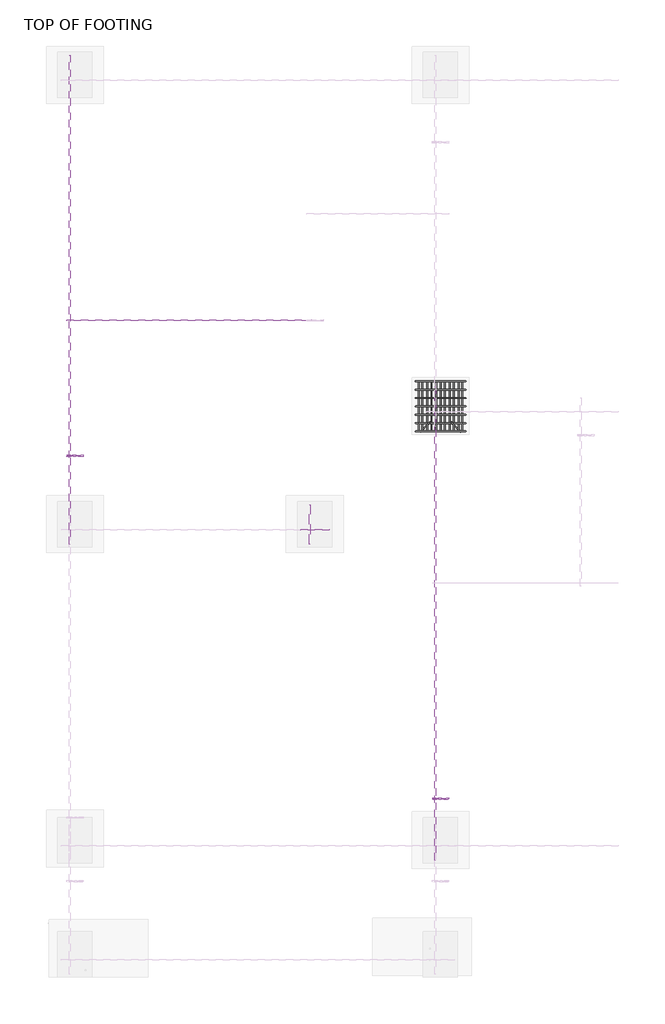
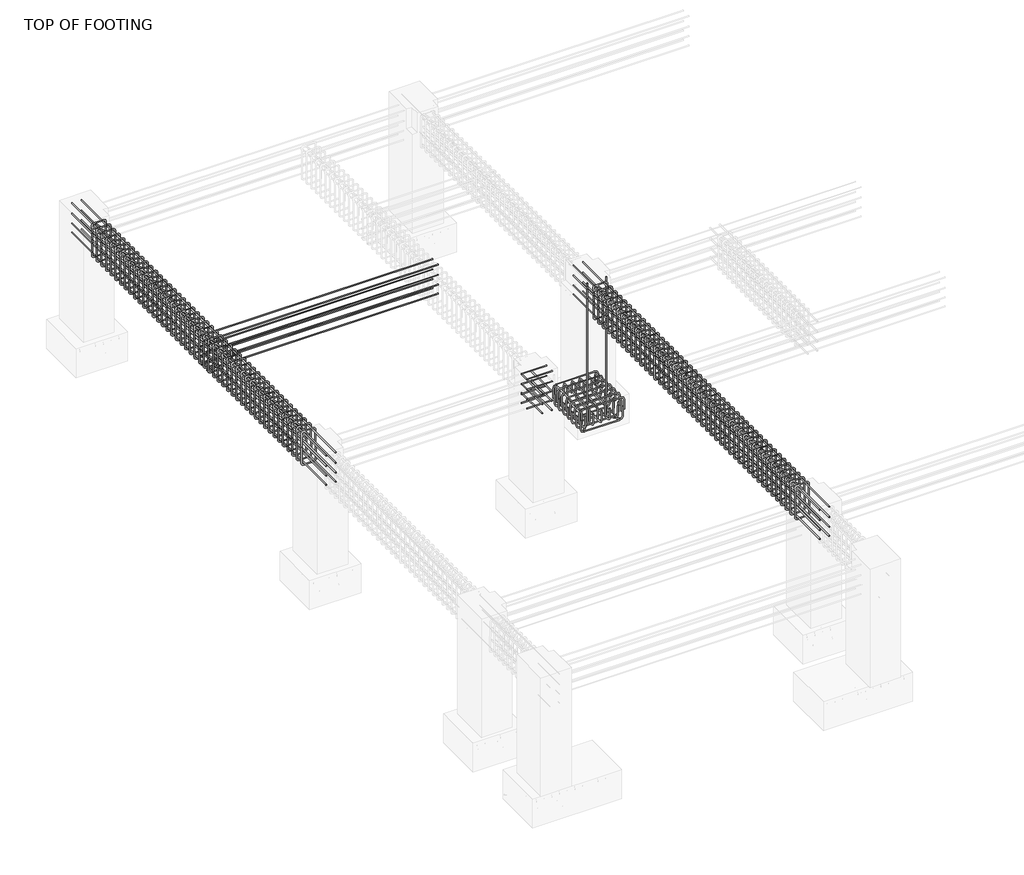
# One storey, part 5 of 8: 27 reinforcing bars.
"""IFC4 building model written with IfcOpenShell, lengths in millimetres."""

from ifc_helpers import new_model, si_unit, point, frame, origin, place, context, project, spatial, polyline, circle_curve, trimmed, segment, composite_curve, source, transform, mapped, element, save
from ifc_brep_helpers import swept_disk

model = new_model("IFC4")

# Units and contexts
model_context = context("Model", 3, world=origin())
ifc_project = project(units=[si_unit("LENGTHUNIT", "METRE", prefix="MILLI")], contexts=[model_context])

# Site, building, storey
site = spatial("IfcSite", under=ifc_project)
building = spatial("IfcBuilding", under=site)
storey = spatial("IfcBuildingStorey", under=building, Name="TOP OF FOOTING", Elevation=-1828.8)

# Reinforcing bars
placement = place(None, origin())
reinforcing_bar_shape = source(origin(), model_context, "Body", "SolidModel", [
    swept_disk(composite_curve([segment(polyline([(-1395.5877818, 5545.6420243, -2021.245224), (-1395.5877818, 5545.6420243, -2168.545224)]), True, "CONTINUOUS"), segment(trimmed(circle_curve(frame((-1441.9377818, 5545.6420243, -2168.545224), z_axis=(0.0, 1.0, 0.0), x_axis=(46.350000000000136, 0.0, 0.0)), 46.35), [point((-1395.5877818, 5545.6420243, -2168.545224))], [point((-1441.9377818, 5545.6420243, -2214.895224))], True, "CARTESIAN"), True, "CONTINUOUS"), segment(polyline([(-1441.9377818, 5545.6420243, -2214.895224), (-1962.8758647, 5545.6420243, -2214.895224)]), True, "CONTINUOUS"), segment(trimmed(circle_curve(frame((-1962.8758647, 5545.6420243, -2168.545224), z_axis=(0.0, 1.0, 0.0), x_axis=(0.0, 0.0, -46.34999999999991)), 46.35), [point((-1962.8758647, 5545.6420243, -2214.895224))], [point((-2009.2258647, 5545.6420243, -2168.545224))], True, "CARTESIAN"), True, "CONTINUOUS"), segment(polyline([(-2009.2258647, 5545.6420243, -2168.545224), (-2009.2258647, 5545.6420243, -2021.245224)]), True, "CONTINUOUS")], self_intersect=False), 6.35),
])
element("IfcReinforcingBar", 1, at=placement, inside=storey, context=model_context, shape_type="MappedRepresentation", body=[
    mapped(reinforcing_bar_shape, transform((0.0, 0.0, 0.0), x_axis=(1.0, 0.0, 0.0), y_axis=(0.0, 1.0, 0.0), z_axis=(0.0, 0.0, 1.0))),
    mapped(reinforcing_bar_shape, transform((0.0, -109.55, 0.0), x_axis=(1.0, 0.0, 0.0), y_axis=(0.0, 1.0, 0.0), z_axis=(0.0, 0.0, 1.0))),
    mapped(reinforcing_bar_shape, transform((0.0, -219.1, 0.0), x_axis=(1.0, 0.0, 0.0), y_axis=(0.0, 1.0, 0.0), z_axis=(0.0, 0.0, 1.0))),
    mapped(reinforcing_bar_shape, transform((0.0, -328.65, 0.0), x_axis=(1.0, 0.0, 0.0), y_axis=(0.0, 1.0, 0.0), z_axis=(0.0, 0.0, 1.0))),
    mapped(reinforcing_bar_shape, transform((0.0, -438.2, 0.0), x_axis=(1.0, 0.0, 0.0), y_axis=(0.0, 1.0, 0.0), z_axis=(0.0, 0.0, 1.0))),
    mapped(reinforcing_bar_shape, transform((0.0, -547.75, 0.0), x_axis=(1.0, 0.0, 0.0), y_axis=(0.0, 1.0, 0.0), z_axis=(0.0, 0.0, 1.0))),
    mapped(reinforcing_bar_shape, transform((0.0, -657.3, 0.0), x_axis=(1.0, 0.0, 0.0), y_axis=(0.0, 1.0, 0.0), z_axis=(0.0, 0.0, 1.0))),
])
reinforcing_bar_2_shape = source(origin(), model_context, "Body", "SolidModel", [
    swept_disk(composite_curve([segment(polyline([(-2031.1461367, 5545.6420243, -2068.8), (-2031.1461367, 5545.6420243, -1921.5)]), True, "CONTINUOUS"), segment(trimmed(circle_curve(frame((-1984.7961367, 5545.6420243, -1921.5), z_axis=(0.0, 1.0, 0.0), x_axis=(-46.34999999999991, 0.0, 0.0)), 46.35), [point((-2031.1461367, 5545.6420243, -1921.5))], [point((-1984.7961367, 5545.6420243, -1875.15))], True, "CARTESIAN"), True, "CONTINUOUS"), segment(polyline([(-1984.7961367, 5545.6420243, -1875.15), (-1420.1961367, 5545.6420243, -1875.15)]), True, "CONTINUOUS"), segment(trimmed(circle_curve(frame((-1420.1961367, 5545.6420243, -1921.5), z_axis=(0.0, 1.0, 0.0), x_axis=(0.0, 0.0, 46.34999999999991)), 46.35), [point((-1420.1961367, 5545.6420243, -1875.15))], [point((-1373.8461367, 5545.6420243, -1921.5))], True, "CARTESIAN"), True, "CONTINUOUS"), segment(polyline([(-1373.8461367, 5545.6420243, -1921.5), (-1373.8461367, 5545.6420243, -2068.8)]), True, "CONTINUOUS")], self_intersect=False), 6.35),
])
element("IfcReinforcingBar", 2, at=placement, inside=storey, context=model_context, shape_type="MappedRepresentation", body=[
    mapped(reinforcing_bar_2_shape, transform((0.0, 0.0, 0.0), x_axis=(1.0, 0.0, 0.0), y_axis=(0.0, 1.0, 0.0), z_axis=(0.0, 0.0, 1.0))),
    mapped(reinforcing_bar_2_shape, transform((0.0, -109.55, 0.0), x_axis=(1.0, 0.0, 0.0), y_axis=(0.0, 1.0, 0.0), z_axis=(0.0, 0.0, 1.0))),
    mapped(reinforcing_bar_2_shape, transform((0.0, -219.1, 0.0), x_axis=(1.0, 0.0, 0.0), y_axis=(0.0, 1.0, 0.0), z_axis=(0.0, 0.0, 1.0))),
    mapped(reinforcing_bar_2_shape, transform((0.0, -328.65, 0.0), x_axis=(1.0, 0.0, 0.0), y_axis=(0.0, 1.0, 0.0), z_axis=(0.0, 0.0, 1.0))),
    mapped(reinforcing_bar_2_shape, transform((0.0, -438.2, 0.0), x_axis=(1.0, 0.0, 0.0), y_axis=(0.0, 1.0, 0.0), z_axis=(0.0, 0.0, 1.0))),
    mapped(reinforcing_bar_2_shape, transform((0.0, -547.75, 0.0), x_axis=(1.0, 0.0, 0.0), y_axis=(0.0, 1.0, 0.0), z_axis=(0.0, 0.0, 1.0))),
    mapped(reinforcing_bar_2_shape, transform((0.0, -657.3, 0.0), x_axis=(1.0, 0.0, 0.0), y_axis=(0.0, 1.0, 0.0), z_axis=(0.0, 0.0, 1.0))),
])
reinforcing_bar_3_shape = source(origin(), model_context, "Body", "SolidModel", [
    swept_disk(composite_curve([segment(polyline([(-1419.0253093, 5545.6420243, -2080.9203068), (-1419.0253093, 5545.6420243, -1933.6203068)]), True, "CONTINUOUS"), segment(trimmed(circle_curve(frame((-1419.0253093, 5499.2920243, -1933.6203068), z_axis=(1.0, 0.0, 0.0), x_axis=(0.0, 46.350000000000364, 0.0)), 46.35), [point((-1419.0253093, 5545.6420243, -1933.6203068))], [point((-1419.0253093, 5499.2920243, -1887.2703068))], True, "CARTESIAN"), True, "CONTINUOUS"), segment(polyline([(-1419.0253093, 5499.2920243, -1887.2703068), (-1419.0253093, 4934.6920243, -1887.2703068)]), True, "CONTINUOUS"), segment(trimmed(circle_curve(frame((-1419.0253093, 4934.6920243, -1933.6203068), z_axis=(1.0, 0.0, 0.0), x_axis=(0.0, 0.0, 46.34999999999991)), 46.35), [point((-1419.0253093, 4934.6920243, -1887.2703068))], [point((-1419.0253093, 4888.3420243, -1933.6203068))], True, "CARTESIAN"), True, "CONTINUOUS"), segment(polyline([(-1419.0253093, 4888.3420243, -1933.6203068), (-1419.0253093, 4888.3420243, -2080.9203068)]), True, "CONTINUOUS")], self_intersect=False), 6.35),
])
element("IfcReinforcingBar", 3, at=placement, inside=storey, context=model_context, shape_type="MappedRepresentation", body=[
    mapped(reinforcing_bar_3_shape, transform((0.0, 0.0, 0.0), x_axis=(1.0, 0.0, 0.0), y_axis=(0.0, 1.0, 0.0), z_axis=(0.0, 0.0, 1.0))),
    mapped(reinforcing_bar_3_shape, transform((-113.9683653, 0.0, 0.0), x_axis=(1.0, 0.0, 0.0), y_axis=(0.0, 1.0, 0.0), z_axis=(0.0, 0.0, 1.0))),
    mapped(reinforcing_bar_3_shape, transform((-227.9367307, 0.0, 0.0), x_axis=(1.0, 0.0, 0.0), y_axis=(0.0, 1.0, 0.0), z_axis=(0.0, 0.0, 1.0))),
    mapped(reinforcing_bar_3_shape, transform((-341.905096, 0.0, 0.0), x_axis=(1.0, 0.0, 0.0), y_axis=(0.0, 1.0, 0.0), z_axis=(0.0, 0.0, 1.0))),
    mapped(reinforcing_bar_3_shape, transform((-455.8734613, 0.0, 0.0), x_axis=(1.0, 0.0, 0.0), y_axis=(0.0, 1.0, 0.0), z_axis=(0.0, 0.0, 1.0))),
    mapped(reinforcing_bar_3_shape, transform((-569.8418267, 0.0, 0.0), x_axis=(1.0, 0.0, 0.0), y_axis=(0.0, 1.0, 0.0), z_axis=(0.0, 0.0, 1.0))),
])
reinforcing_bar_4_shape = source(origin(), model_context, "Body", "SolidModel", [
    swept_disk(composite_curve([segment(polyline([(-1941.3656272, 5545.6420243, -1984.9681267), (-1941.3656272, 5545.6420243, -2132.2681267)]), True, "CONTINUOUS"), segment(trimmed(circle_curve(frame((-1941.3656272, 5499.2920243, -2132.2681267), z_axis=(-1.0, 0.0, 0.0), x_axis=(0.0, 46.350000000000364, 0.0)), 46.35), [point((-1941.3656272, 5545.6420243, -2132.2681267))], [point((-1941.3656272, 5499.2920243, -2178.6181267))], True, "CARTESIAN"), True, "CONTINUOUS"), segment(polyline([(-1941.3656272, 5499.2920243, -2178.6181267), (-1941.3656272, 4934.6920243, -2178.6181267)]), True, "CONTINUOUS"), segment(trimmed(circle_curve(frame((-1941.3656272, 4934.6920243, -2132.2681267), z_axis=(-1.0, 0.0, 0.0), x_axis=(0.0, 0.0, -46.350000000000364)), 46.35), [point((-1941.3656272, 4934.6920243, -2178.6181267))], [point((-1941.3656272, 4888.3420243, -2132.2681267))], True, "CARTESIAN"), True, "CONTINUOUS"), segment(polyline([(-1941.3656272, 4888.3420243, -2132.2681267), (-1941.3656272, 4888.3420243, -1984.9681267)]), True, "CONTINUOUS")], self_intersect=False), 6.35),
])
element("IfcReinforcingBar", 4, at=placement, inside=storey, context=model_context, shape_type="MappedRepresentation", body=[
    mapped(reinforcing_bar_4_shape, transform((0.0, 0.0, 0.0), x_axis=(1.0, 0.0, 0.0), y_axis=(0.0, 1.0, 0.0), z_axis=(0.0, 0.0, 1.0))),
    mapped(reinforcing_bar_4_shape, transform((119.2770606, 0.0, 0.0), x_axis=(1.0, 0.0, 0.0), y_axis=(0.0, 1.0, 0.0), z_axis=(0.0, 0.0, 1.0))),
    mapped(reinforcing_bar_4_shape, transform((238.5541211, 0.0, 0.0), x_axis=(1.0, 0.0, 0.0), y_axis=(0.0, 1.0, 0.0), z_axis=(0.0, 0.0, 1.0))),
    mapped(reinforcing_bar_4_shape, transform((357.8311817, 0.0, 0.0), x_axis=(1.0, 0.0, 0.0), y_axis=(0.0, 1.0, 0.0), z_axis=(0.0, 0.0, 1.0))),
    mapped(reinforcing_bar_4_shape, transform((477.1082423, 0.0, 0.0), x_axis=(1.0, 0.0, 0.0), y_axis=(0.0, 1.0, 0.0), z_axis=(0.0, 0.0, 1.0))),
])
element("IfcReinforcingBar", 5, at=placement, inside=storey, context=model_context, shape_type="SolidModel", body=[
    swept_disk(composite_curve([segment(polyline([(-1968.0144002, 4882.6300935, -2192.6897268), (-1873.5395717, 4977.1049221, -2192.6897268)]), True, "CONTINUOUS"), segment(trimmed(circle_curve(frame((-1873.5395717, 4977.1049221, -2146.3397268), z_axis=(0.7071067811865476, -0.7071067811865475, 0.0), x_axis=(0.0, 0.0, -46.34999999999991)), 46.35), [point((-1873.5395717, 4977.1049221, -2192.6897268))], [point((-1840.7651723, 5009.8793214, -2146.3397268))], True, "CARTESIAN"), True, "CONTINUOUS"), segment(polyline([(-1840.7651723, 5009.8793214, -2146.3397268), (-1840.7651723, 5009.8793214, -40.0)]), True, "CONTINUOUS")], self_intersect=False), 6.35),
])
element("IfcReinforcingBar", 6, at=placement, inside=storey, context=model_context, shape_type="SolidModel", body=[
    swept_disk(composite_curve([segment(polyline([(-1436.9778732, 4882.6300935, -2192.6897268), (-1531.4527018, 4977.1049221, -2192.6897268)]), True, "CONTINUOUS"), segment(trimmed(circle_curve(frame((-1531.4527018, 4977.1049221, -2146.3397268), z_axis=(0.7071067811865753, 0.7071067811865197, 0.0), x_axis=(0.0, 0.0, -46.34999999999991)), 46.35), [point((-1531.4527018, 4977.1049221, -2192.6897268))], [point((-1564.2271011, 5009.8793214, -2146.3397268))], True, "CARTESIAN"), True, "CONTINUOUS"), segment(polyline([(-1564.2271011, 5009.8793214, -2146.3397268), (-1564.2271011, 5009.8793214, -40.0)]), True, "CONTINUOUS")], self_intersect=False), 6.35),
])
reinforcing_bar_5_shape = source(origin(), model_context, "Body", "SolidModel", [
    swept_disk(composite_curve([segment(polyline([(-6496.8847762, 9260.6420243, -111.2757654), (-6552.6283391, 9260.6420243, -55.5322024)]), True, "CONTINUOUS"), segment(trimmed(circle_curve(frame((-6574.7961367, 9260.6420243, -77.7), z_axis=(0.0, -1.0, 0.0), x_axis=(22.167797600000085, 0.0, 22.1677976)), 31.35), [point((-6552.6283391, 9260.6420243, -55.5322024))], [point((-6606.1461367, 9260.6420243, -77.7))], True, "CARTESIAN"), True, "CONTINUOUS"), segment(polyline([(-6606.1461367, 9260.6420243, -77.7), (-6606.1461367, 9260.6420243, -522.3)]), True, "CONTINUOUS"), segment(trimmed(circle_curve(frame((-6574.7961367, 9260.6420243, -522.3), z_axis=(0.0, -1.0, 0.0), x_axis=(-31.350000000000364, 0.0, 0.0)), 31.35), [point((-6606.1461367, 9260.6420243, -522.3))], [point((-6574.7961367, 9260.6420243, -553.65))], True, "CARTESIAN"), True, "CONTINUOUS"), segment(polyline([(-6574.7961367, 9260.6420243, -553.65), (-6430.1961367, 9260.6420243, -553.65)]), True, "CONTINUOUS"), segment(trimmed(circle_curve(frame((-6430.1961367, 9261.4266099, -522.3098193), z_axis=(0.0, -0.9996867842138424, 0.025026655153786322), x_axis=(0.0, -0.784585600000355, -31.34018070000002)), 31.35), [point((-6430.1961367, 9260.6420243, -553.65))], [point((-6398.8461367, 9261.4266099, -522.3098193))], True, "CARTESIAN"), True, "CONTINUOUS"), segment(polyline([(-6398.8461367, 9261.4266099, -522.3098193), (-6398.8461367, 9272.5574386, -77.6901807)]), True, "CONTINUOUS"), segment(trimmed(circle_curve(frame((-6430.1961367, 9272.5574386, -77.6901807), z_axis=(0.0, -0.9996867842138424, 0.025026655153786322), x_axis=(31.350000000000364, 0.0, 0.0)), 31.35), [point((-6398.8461367, 9272.5574386, -77.6901807))], [point((-6430.1961367, 9273.3420243, -46.35))], True, "CARTESIAN"), True, "CONTINUOUS"), segment(polyline([(-6430.1961367, 9273.3420243, -46.35), (-6574.7961367, 9273.3420243, -46.35)]), True, "CONTINUOUS"), segment(trimmed(circle_curve(frame((-6574.7961367, 9273.3420243, -77.7), z_axis=(0.0, -1.0, 0.0), x_axis=(0.0, 0.0, 31.35)), 31.35), [point((-6574.7961367, 9273.3420243, -46.35))], [point((-6596.9639343, 9273.3420243, -99.8677976))], True, "CARTESIAN"), True, "CONTINUOUS"), segment(polyline([(-6596.9639343, 9273.3420243, -99.8677976), (-6541.2203714, 9273.3420243, -155.6113605)]), True, "CONTINUOUS")], self_intersect=False), 6.35),
])
element("IfcReinforcingBar", 7, at=placement, inside=storey, context=model_context, shape_type="MappedRepresentation", body=[
    mapped(reinforcing_bar_5_shape, transform((0.0, 0.0, 0.0), x_axis=(1.0, 0.0, 0.0), y_axis=(0.0, 1.0, 0.0), z_axis=(0.0, 0.0, 1.0))),
    mapped(reinforcing_bar_5_shape, transform((0.0, -117.4955556, 0.0), x_axis=(1.0, 0.0, 0.0), y_axis=(0.0, 1.0, 0.0), z_axis=(0.0, 0.0, 1.0))),
    mapped(reinforcing_bar_5_shape, transform((0.0, -234.9911111, 0.0), x_axis=(1.0, 0.0, 0.0), y_axis=(0.0, 1.0, 0.0), z_axis=(0.0, 0.0, 1.0))),
    mapped(reinforcing_bar_5_shape, transform((0.0, -352.4866667, 0.0), x_axis=(1.0, 0.0, 0.0), y_axis=(0.0, 1.0, 0.0), z_axis=(0.0, 0.0, 1.0))),
    mapped(reinforcing_bar_5_shape, transform((0.0, -469.9822222, 0.0), x_axis=(1.0, 0.0, 0.0), y_axis=(0.0, 1.0, 0.0), z_axis=(0.0, 0.0, 1.0))),
    mapped(reinforcing_bar_5_shape, transform((0.0, -587.4777778, 0.0), x_axis=(1.0, 0.0, 0.0), y_axis=(0.0, 1.0, 0.0), z_axis=(0.0, 0.0, 1.0))),
    mapped(reinforcing_bar_5_shape, transform((0.0, -704.9733333, 0.0), x_axis=(1.0, 0.0, 0.0), y_axis=(0.0, 1.0, 0.0), z_axis=(0.0, 0.0, 1.0))),
    mapped(reinforcing_bar_5_shape, transform((0.0, -822.4688889, 0.0), x_axis=(1.0, 0.0, 0.0), y_axis=(0.0, 1.0, 0.0), z_axis=(0.0, 0.0, 1.0))),
    mapped(reinforcing_bar_5_shape, transform((0.0, -939.9644444, 0.0), x_axis=(1.0, 0.0, 0.0), y_axis=(0.0, 1.0, 0.0), z_axis=(0.0, 0.0, 1.0))),
    mapped(reinforcing_bar_5_shape, transform((0.0, -1057.46, 0.0), x_axis=(1.0, 0.0, 0.0), y_axis=(0.0, 1.0, 0.0), z_axis=(0.0, 0.0, 1.0))),
    mapped(reinforcing_bar_5_shape, transform((0.0, -1174.9555556, 0.0), x_axis=(1.0, 0.0, 0.0), y_axis=(0.0, 1.0, 0.0), z_axis=(0.0, 0.0, 1.0))),
    mapped(reinforcing_bar_5_shape, transform((0.0, -1292.4511111, 0.0), x_axis=(1.0, 0.0, 0.0), y_axis=(0.0, 1.0, 0.0), z_axis=(0.0, 0.0, 1.0))),
    mapped(reinforcing_bar_5_shape, transform((0.0, -1409.9466667, 0.0), x_axis=(1.0, 0.0, 0.0), y_axis=(0.0, 1.0, 0.0), z_axis=(0.0, 0.0, 1.0))),
    mapped(reinforcing_bar_5_shape, transform((0.0, -1527.4422222, 0.0), x_axis=(1.0, 0.0, 0.0), y_axis=(0.0, 1.0, 0.0), z_axis=(0.0, 0.0, 1.0))),
    mapped(reinforcing_bar_5_shape, transform((0.0, -1644.9377778, 0.0), x_axis=(1.0, 0.0, 0.0), y_axis=(0.0, 1.0, 0.0), z_axis=(0.0, 0.0, 1.0))),
    mapped(reinforcing_bar_5_shape, transform((0.0, -1762.4333333, 0.0), x_axis=(1.0, 0.0, 0.0), y_axis=(0.0, 1.0, 0.0), z_axis=(0.0, 0.0, 1.0))),
    mapped(reinforcing_bar_5_shape, transform((0.0, -1879.9288889, 0.0), x_axis=(1.0, 0.0, 0.0), y_axis=(0.0, 1.0, 0.0), z_axis=(0.0, 0.0, 1.0))),
    mapped(reinforcing_bar_5_shape, transform((0.0, -1997.4244444, 0.0), x_axis=(1.0, 0.0, 0.0), y_axis=(0.0, 1.0, 0.0), z_axis=(0.0, 0.0, 1.0))),
    mapped(reinforcing_bar_5_shape, transform((0.0, -2114.92, 0.0), x_axis=(1.0, 0.0, 0.0), y_axis=(0.0, 1.0, 0.0), z_axis=(0.0, 0.0, 1.0))),
    mapped(reinforcing_bar_5_shape, transform((0.0, -2232.4155556, 0.0), x_axis=(1.0, 0.0, 0.0), y_axis=(0.0, 1.0, 0.0), z_axis=(0.0, 0.0, 1.0))),
    mapped(reinforcing_bar_5_shape, transform((0.0, -2349.9111111, 0.0), x_axis=(1.0, 0.0, 0.0), y_axis=(0.0, 1.0, 0.0), z_axis=(0.0, 0.0, 1.0))),
    mapped(reinforcing_bar_5_shape, transform((0.0, -2467.4066667, 0.0), x_axis=(1.0, 0.0, 0.0), y_axis=(0.0, 1.0, 0.0), z_axis=(0.0, 0.0, 1.0))),
    mapped(reinforcing_bar_5_shape, transform((0.0, -2584.9022222, 0.0), x_axis=(1.0, 0.0, 0.0), y_axis=(0.0, 1.0, 0.0), z_axis=(0.0, 0.0, 1.0))),
    mapped(reinforcing_bar_5_shape, transform((0.0, -2702.3977778, 0.0), x_axis=(1.0, 0.0, 0.0), y_axis=(0.0, 1.0, 0.0), z_axis=(0.0, 0.0, 1.0))),
    mapped(reinforcing_bar_5_shape, transform((0.0, -2819.8933333, 0.0), x_axis=(1.0, 0.0, 0.0), y_axis=(0.0, 1.0, 0.0), z_axis=(0.0, 0.0, 1.0))),
    mapped(reinforcing_bar_5_shape, transform((0.0, -2937.3888889, 0.0), x_axis=(1.0, 0.0, 0.0), y_axis=(0.0, 1.0, 0.0), z_axis=(0.0, 0.0, 1.0))),
    mapped(reinforcing_bar_5_shape, transform((0.0, -3054.8844444, 0.0), x_axis=(1.0, 0.0, 0.0), y_axis=(0.0, 1.0, 0.0), z_axis=(0.0, 0.0, 1.0))),
    mapped(reinforcing_bar_5_shape, transform((0.0, -3172.38, 0.0), x_axis=(1.0, 0.0, 0.0), y_axis=(0.0, 1.0, 0.0), z_axis=(0.0, 0.0, 1.0))),
    mapped(reinforcing_bar_5_shape, transform((0.0, -3289.8755556, 0.0), x_axis=(1.0, 0.0, 0.0), y_axis=(0.0, 1.0, 0.0), z_axis=(0.0, 0.0, 1.0))),
    mapped(reinforcing_bar_5_shape, transform((0.0, -3407.3711111, 0.0), x_axis=(1.0, 0.0, 0.0), y_axis=(0.0, 1.0, 0.0), z_axis=(0.0, 0.0, 1.0))),
    mapped(reinforcing_bar_5_shape, transform((0.0, -3524.8666667, 0.0), x_axis=(1.0, 0.0, 0.0), y_axis=(0.0, 1.0, 0.0), z_axis=(0.0, 0.0, 1.0))),
    mapped(reinforcing_bar_5_shape, transform((0.0, -3642.3622222, 0.0), x_axis=(1.0, 0.0, 0.0), y_axis=(0.0, 1.0, 0.0), z_axis=(0.0, 0.0, 1.0))),
    mapped(reinforcing_bar_5_shape, transform((0.0, -3759.8577778, 0.0), x_axis=(1.0, 0.0, 0.0), y_axis=(0.0, 1.0, 0.0), z_axis=(0.0, 0.0, 1.0))),
    mapped(reinforcing_bar_5_shape, transform((0.0, -3877.3533333, 0.0), x_axis=(1.0, 0.0, 0.0), y_axis=(0.0, 1.0, 0.0), z_axis=(0.0, 0.0, 1.0))),
    mapped(reinforcing_bar_5_shape, transform((0.0, -3994.8488889, 0.0), x_axis=(1.0, 0.0, 0.0), y_axis=(0.0, 1.0, 0.0), z_axis=(0.0, 0.0, 1.0))),
    mapped(reinforcing_bar_5_shape, transform((0.0, -4112.3444444, 0.0), x_axis=(1.0, 0.0, 0.0), y_axis=(0.0, 1.0, 0.0), z_axis=(0.0, 0.0, 1.0))),
    mapped(reinforcing_bar_5_shape, transform((0.0, -4229.84, 0.0), x_axis=(1.0, 0.0, 0.0), y_axis=(0.0, 1.0, 0.0), z_axis=(0.0, 0.0, 1.0))),
    mapped(reinforcing_bar_5_shape, transform((0.0, -4347.3355556, 0.0), x_axis=(1.0, 0.0, 0.0), y_axis=(0.0, 1.0, 0.0), z_axis=(0.0, 0.0, 1.0))),
    mapped(reinforcing_bar_5_shape, transform((0.0, -4464.8311111, 0.0), x_axis=(1.0, 0.0, 0.0), y_axis=(0.0, 1.0, 0.0), z_axis=(0.0, 0.0, 1.0))),
    mapped(reinforcing_bar_5_shape, transform((0.0, -4582.3266667, 0.0), x_axis=(1.0, 0.0, 0.0), y_axis=(0.0, 1.0, 0.0), z_axis=(0.0, 0.0, 1.0))),
    mapped(reinforcing_bar_5_shape, transform((0.0, -4699.8222222, 0.0), x_axis=(1.0, 0.0, 0.0), y_axis=(0.0, 1.0, 0.0), z_axis=(0.0, 0.0, 1.0))),
    mapped(reinforcing_bar_5_shape, transform((0.0, -4817.3177778, 0.0), x_axis=(1.0, 0.0, 0.0), y_axis=(0.0, 1.0, 0.0), z_axis=(0.0, 0.0, 1.0))),
    mapped(reinforcing_bar_5_shape, transform((0.0, -4934.8133333, 0.0), x_axis=(1.0, 0.0, 0.0), y_axis=(0.0, 1.0, 0.0), z_axis=(0.0, 0.0, 1.0))),
    mapped(reinforcing_bar_5_shape, transform((0.0, -5052.3088889, 0.0), x_axis=(1.0, 0.0, 0.0), y_axis=(0.0, 1.0, 0.0), z_axis=(0.0, 0.0, 1.0))),
    mapped(reinforcing_bar_5_shape, transform((0.0, -5169.8044444, 0.0), x_axis=(1.0, 0.0, 0.0), y_axis=(0.0, 1.0, 0.0), z_axis=(0.0, 0.0, 1.0))),
    mapped(reinforcing_bar_5_shape, transform((0.0, -5287.3, 0.0), x_axis=(1.0, 0.0, 0.0), y_axis=(0.0, 1.0, 0.0), z_axis=(0.0, 0.0, 1.0))),
])
reinforcing_bar_6_shape = source(origin(), model_context, "Body", "SolidModel", [
    swept_disk(composite_curve([segment(polyline([(-6432.8743653, 9826.9920243, -72.7), (-6432.8743653, 3406.9920243, -72.7)]), True, "CONTINUOUS")], self_intersect=False), 6.35),
])
element("IfcReinforcingBar", 8, at=placement, inside=storey, context=model_context, shape_type="MappedRepresentation", body=[
    mapped(reinforcing_bar_6_shape, transform((0.0, 0.0, 0.0), x_axis=(1.0, 0.0, 0.0), y_axis=(0.0, 1.0, 0.0), z_axis=(0.0, 0.0, 1.0))),
    mapped(reinforcing_bar_6_shape, transform((-139.7429418, 0.0, 0.0), x_axis=(1.0, 0.0, 0.0), y_axis=(0.0, 1.0, 0.0), z_axis=(0.0, 0.0, 1.0))),
])
reinforcing_bar_7_shape = source(origin(), model_context, "Body", "SolidModel", [
    swept_disk(composite_curve([segment(polyline([(-6432.8743653, 9826.9920243, -522.7), (-6432.8743653, 3406.9920243, -522.7)]), True, "CONTINUOUS")], self_intersect=False), 6.35),
])
element("IfcReinforcingBar", 9, at=placement, inside=storey, context=model_context, shape_type="MappedRepresentation", body=[
    mapped(reinforcing_bar_7_shape, transform((0.0, 0.0, 0.0), x_axis=(1.0, 0.0, 0.0), y_axis=(0.0, 1.0, 0.0), z_axis=(0.0, 0.0, 1.0))),
    mapped(reinforcing_bar_7_shape, transform((-139.7429418, 0.0, 0.0), x_axis=(1.0, 0.0, 0.0), y_axis=(0.0, 1.0, 0.0), z_axis=(0.0, 0.0, 1.0))),
])
reinforcing_bar_8_shape = source(origin(), model_context, "Body", "SolidModel", [
    swept_disk(composite_curve([segment(polyline([(-6432.8743653, 9826.9920243, -382.7), (-6432.8743653, 3406.9920243, -382.7)]), True, "CONTINUOUS")], self_intersect=False), 6.35),
])
element("IfcReinforcingBar", 10, at=placement, inside=storey, context=model_context, shape_type="MappedRepresentation", body=[
    mapped(reinforcing_bar_8_shape, transform((0.0, 0.0, 0.0), x_axis=(1.0, 0.0, 0.0), y_axis=(0.0, 1.0, 0.0), z_axis=(0.0, 0.0, 1.0))),
    mapped(reinforcing_bar_8_shape, transform((-139.7429418, 0.0, 0.0), x_axis=(1.0, 0.0, 0.0), y_axis=(0.0, 1.0, 0.0), z_axis=(0.0, 0.0, 1.0))),
])
reinforcing_bar_9_shape = source(origin(), model_context, "Body", "SolidModel", [
    swept_disk(composite_curve([segment(polyline([(-6432.8743653, 9826.9920243, -232.7), (-6432.8743653, 3406.9920243, -232.7)]), True, "CONTINUOUS")], self_intersect=False), 6.35),
])
element("IfcReinforcingBar", 11, at=placement, inside=storey, context=model_context, shape_type="MappedRepresentation", body=[
    mapped(reinforcing_bar_9_shape, transform((0.0, 0.0, 0.0), x_axis=(1.0, 0.0, 0.0), y_axis=(0.0, 1.0, 0.0), z_axis=(0.0, 0.0, 1.0))),
    mapped(reinforcing_bar_9_shape, transform((-139.7429418, 0.0, 0.0), x_axis=(1.0, 0.0, 0.0), y_axis=(0.0, 1.0, 0.0), z_axis=(0.0, 0.0, 1.0))),
])
reinforcing_bar_10_shape = source(origin(), model_context, "Body", "SolidModel", [
    swept_disk(composite_curve([segment(polyline([(-1696.8847762, 4910.6420243, -111.2757654), (-1752.6283391, 4910.6420243, -55.5322024)]), True, "CONTINUOUS"), segment(trimmed(circle_curve(frame((-1774.7961367, 4910.6420243, -77.7), z_axis=(0.0, -1.0, 0.0), x_axis=(22.167797600000085, 0.0, 22.1677976)), 31.35), [point((-1752.6283391, 4910.6420243, -55.5322024))], [point((-1806.1461367, 4910.6420243, -77.7))], True, "CARTESIAN"), True, "CONTINUOUS"), segment(polyline([(-1806.1461367, 4910.6420243, -77.7), (-1806.1461367, 4910.6420243, -522.3)]), True, "CONTINUOUS"), segment(trimmed(circle_curve(frame((-1774.7961367, 4910.6420243, -522.3), z_axis=(0.0, -1.0, 0.0), x_axis=(-31.34999999999991, 0.0, 0.0)), 31.35), [point((-1806.1461367, 4910.6420243, -522.3))], [point((-1774.7961367, 4910.6420243, -553.65))], True, "CARTESIAN"), True, "CONTINUOUS"), segment(polyline([(-1774.7961367, 4910.6420243, -553.65), (-1630.1961367, 4910.6420243, -553.65)]), True, "CONTINUOUS"), segment(trimmed(circle_curve(frame((-1630.1961367, 4911.4266099, -522.3098193), z_axis=(0.0, -0.9996867842138424, 0.025026655153786322), x_axis=(0.0, -0.7845855999994455, -31.34018070000002)), 31.35), [point((-1630.1961367, 4910.6420243, -553.65))], [point((-1598.8461367, 4911.4266099, -522.3098193))], True, "CARTESIAN"), True, "CONTINUOUS"), segment(polyline([(-1598.8461367, 4911.4266099, -522.3098193), (-1598.8461367, 4922.5574386, -77.6901807)]), True, "CONTINUOUS"), segment(trimmed(circle_curve(frame((-1630.1961367, 4922.5574386, -77.6901807), z_axis=(0.0, -0.9996867842138424, 0.025026655153786322), x_axis=(31.34999999999991, 0.0, 0.0)), 31.35), [point((-1598.8461367, 4922.5574386, -77.6901807))], [point((-1630.1961367, 4923.3420243, -46.35))], True, "CARTESIAN"), True, "CONTINUOUS"), segment(polyline([(-1630.1961367, 4923.3420243, -46.35), (-1774.7961367, 4923.3420243, -46.35)]), True, "CONTINUOUS"), segment(trimmed(circle_curve(frame((-1774.7961367, 4923.3420243, -77.7), z_axis=(0.0, -1.0, 0.0), x_axis=(0.0, 0.0, 31.35)), 31.35), [point((-1774.7961367, 4923.3420243, -46.35))], [point((-1796.9639343, 4923.3420243, -99.8677976))], True, "CARTESIAN"), True, "CONTINUOUS"), segment(polyline([(-1796.9639343, 4923.3420243, -99.8677976), (-1741.2203714, 4923.3420243, -155.6113605)]), True, "CONTINUOUS")], self_intersect=False), 6.35),
])
element("IfcReinforcingBar", 12, at=placement, inside=storey, context=model_context, shape_type="MappedRepresentation", body=[
    mapped(reinforcing_bar_10_shape, transform((0.0, 0.0, 0.0), x_axis=(1.0, 0.0, 0.0), y_axis=(0.0, 1.0, 0.0), z_axis=(0.0, 0.0, 1.0))),
    mapped(reinforcing_bar_10_shape, transform((0.0, -118.3093023, 0.0), x_axis=(1.0, 0.0, 0.0), y_axis=(0.0, 1.0, 0.0), z_axis=(0.0, 0.0, 1.0))),
    mapped(reinforcing_bar_10_shape, transform((0.0, -236.6186047, 0.0), x_axis=(1.0, 0.0, 0.0), y_axis=(0.0, 1.0, 0.0), z_axis=(0.0, 0.0, 1.0))),
    mapped(reinforcing_bar_10_shape, transform((0.0, -354.927907, 0.0), x_axis=(1.0, 0.0, 0.0), y_axis=(0.0, 1.0, 0.0), z_axis=(0.0, 0.0, 1.0))),
    mapped(reinforcing_bar_10_shape, transform((0.0, -473.2372093, 0.0), x_axis=(1.0, 0.0, 0.0), y_axis=(0.0, 1.0, 0.0), z_axis=(0.0, 0.0, 1.0))),
    mapped(reinforcing_bar_10_shape, transform((0.0, -591.5465116, 0.0), x_axis=(1.0, 0.0, 0.0), y_axis=(0.0, 1.0, 0.0), z_axis=(0.0, 0.0, 1.0))),
    mapped(reinforcing_bar_10_shape, transform((0.0, -709.855814, 0.0), x_axis=(1.0, 0.0, 0.0), y_axis=(0.0, 1.0, 0.0), z_axis=(0.0, 0.0, 1.0))),
    mapped(reinforcing_bar_10_shape, transform((0.0, -828.1651163, 0.0), x_axis=(1.0, 0.0, 0.0), y_axis=(0.0, 1.0, 0.0), z_axis=(0.0, 0.0, 1.0))),
    mapped(reinforcing_bar_10_shape, transform((0.0, -946.4744186, 0.0), x_axis=(1.0, 0.0, 0.0), y_axis=(0.0, 1.0, 0.0), z_axis=(0.0, 0.0, 1.0))),
    mapped(reinforcing_bar_10_shape, transform((0.0, -1064.7837209, 0.0), x_axis=(1.0, 0.0, 0.0), y_axis=(0.0, 1.0, 0.0), z_axis=(0.0, 0.0, 1.0))),
    mapped(reinforcing_bar_10_shape, transform((0.0, -1183.0930233, 0.0), x_axis=(1.0, 0.0, 0.0), y_axis=(0.0, 1.0, 0.0), z_axis=(0.0, 0.0, 1.0))),
    mapped(reinforcing_bar_10_shape, transform((0.0, -1301.4023256, 0.0), x_axis=(1.0, 0.0, 0.0), y_axis=(0.0, 1.0, 0.0), z_axis=(0.0, 0.0, 1.0))),
    mapped(reinforcing_bar_10_shape, transform((0.0, -1419.7116279, 0.0), x_axis=(1.0, 0.0, 0.0), y_axis=(0.0, 1.0, 0.0), z_axis=(0.0, 0.0, 1.0))),
    mapped(reinforcing_bar_10_shape, transform((0.0, -1538.0209302, 0.0), x_axis=(1.0, 0.0, 0.0), y_axis=(0.0, 1.0, 0.0), z_axis=(0.0, 0.0, 1.0))),
    mapped(reinforcing_bar_10_shape, transform((0.0, -1656.3302326, 0.0), x_axis=(1.0, 0.0, 0.0), y_axis=(0.0, 1.0, 0.0), z_axis=(0.0, 0.0, 1.0))),
    mapped(reinforcing_bar_10_shape, transform((0.0, -1774.6395349, 0.0), x_axis=(1.0, 0.0, 0.0), y_axis=(0.0, 1.0, 0.0), z_axis=(0.0, 0.0, 1.0))),
    mapped(reinforcing_bar_10_shape, transform((0.0, -1892.9488372, 0.0), x_axis=(1.0, 0.0, 0.0), y_axis=(0.0, 1.0, 0.0), z_axis=(0.0, 0.0, 1.0))),
    mapped(reinforcing_bar_10_shape, transform((0.0, -2011.2581395, 0.0), x_axis=(1.0, 0.0, 0.0), y_axis=(0.0, 1.0, 0.0), z_axis=(0.0, 0.0, 1.0))),
    mapped(reinforcing_bar_10_shape, transform((0.0, -2129.5674419, 0.0), x_axis=(1.0, 0.0, 0.0), y_axis=(0.0, 1.0, 0.0), z_axis=(0.0, 0.0, 1.0))),
    mapped(reinforcing_bar_10_shape, transform((0.0, -2247.8767442, 0.0), x_axis=(1.0, 0.0, 0.0), y_axis=(0.0, 1.0, 0.0), z_axis=(0.0, 0.0, 1.0))),
    mapped(reinforcing_bar_10_shape, transform((0.0, -2366.1860465, 0.0), x_axis=(1.0, 0.0, 0.0), y_axis=(0.0, 1.0, 0.0), z_axis=(0.0, 0.0, 1.0))),
    mapped(reinforcing_bar_10_shape, transform((0.0, -2484.4953488, 0.0), x_axis=(1.0, 0.0, 0.0), y_axis=(0.0, 1.0, 0.0), z_axis=(0.0, 0.0, 1.0))),
    mapped(reinforcing_bar_10_shape, transform((0.0, -2602.8046512, 0.0), x_axis=(1.0, 0.0, 0.0), y_axis=(0.0, 1.0, 0.0), z_axis=(0.0, 0.0, 1.0))),
    mapped(reinforcing_bar_10_shape, transform((0.0, -2721.1139535, 0.0), x_axis=(1.0, 0.0, 0.0), y_axis=(0.0, 1.0, 0.0), z_axis=(0.0, 0.0, 1.0))),
    mapped(reinforcing_bar_10_shape, transform((0.0, -2839.4232558, 0.0), x_axis=(1.0, 0.0, 0.0), y_axis=(0.0, 1.0, 0.0), z_axis=(0.0, 0.0, 1.0))),
    mapped(reinforcing_bar_10_shape, transform((0.0, -2957.7325581, 0.0), x_axis=(1.0, 0.0, 0.0), y_axis=(0.0, 1.0, 0.0), z_axis=(0.0, 0.0, 1.0))),
    mapped(reinforcing_bar_10_shape, transform((0.0, -3076.0418605, 0.0), x_axis=(1.0, 0.0, 0.0), y_axis=(0.0, 1.0, 0.0), z_axis=(0.0, 0.0, 1.0))),
    mapped(reinforcing_bar_10_shape, transform((0.0, -3194.3511628, 0.0), x_axis=(1.0, 0.0, 0.0), y_axis=(0.0, 1.0, 0.0), z_axis=(0.0, 0.0, 1.0))),
    mapped(reinforcing_bar_10_shape, transform((0.0, -3312.6604651, 0.0), x_axis=(1.0, 0.0, 0.0), y_axis=(0.0, 1.0, 0.0), z_axis=(0.0, 0.0, 1.0))),
    mapped(reinforcing_bar_10_shape, transform((0.0, -3430.9697674, 0.0), x_axis=(1.0, 0.0, 0.0), y_axis=(0.0, 1.0, 0.0), z_axis=(0.0, 0.0, 1.0))),
    mapped(reinforcing_bar_10_shape, transform((0.0, -3549.2790698, 0.0), x_axis=(1.0, 0.0, 0.0), y_axis=(0.0, 1.0, 0.0), z_axis=(0.0, 0.0, 1.0))),
    mapped(reinforcing_bar_10_shape, transform((0.0, -3667.5883721, 0.0), x_axis=(1.0, 0.0, 0.0), y_axis=(0.0, 1.0, 0.0), z_axis=(0.0, 0.0, 1.0))),
    mapped(reinforcing_bar_10_shape, transform((0.0, -3785.8976744, 0.0), x_axis=(1.0, 0.0, 0.0), y_axis=(0.0, 1.0, 0.0), z_axis=(0.0, 0.0, 1.0))),
    mapped(reinforcing_bar_10_shape, transform((0.0, -3904.2069767, 0.0), x_axis=(1.0, 0.0, 0.0), y_axis=(0.0, 1.0, 0.0), z_axis=(0.0, 0.0, 1.0))),
    mapped(reinforcing_bar_10_shape, transform((0.0, -4022.5162791, 0.0), x_axis=(1.0, 0.0, 0.0), y_axis=(0.0, 1.0, 0.0), z_axis=(0.0, 0.0, 1.0))),
    mapped(reinforcing_bar_10_shape, transform((0.0, -4140.8255814, 0.0), x_axis=(1.0, 0.0, 0.0), y_axis=(0.0, 1.0, 0.0), z_axis=(0.0, 0.0, 1.0))),
    mapped(reinforcing_bar_10_shape, transform((0.0, -4259.1348837, 0.0), x_axis=(1.0, 0.0, 0.0), y_axis=(0.0, 1.0, 0.0), z_axis=(0.0, 0.0, 1.0))),
    mapped(reinforcing_bar_10_shape, transform((0.0, -4377.444186, 0.0), x_axis=(1.0, 0.0, 0.0), y_axis=(0.0, 1.0, 0.0), z_axis=(0.0, 0.0, 1.0))),
    mapped(reinforcing_bar_10_shape, transform((0.0, -4495.7534884, 0.0), x_axis=(1.0, 0.0, 0.0), y_axis=(0.0, 1.0, 0.0), z_axis=(0.0, 0.0, 1.0))),
    mapped(reinforcing_bar_10_shape, transform((0.0, -4614.0627907, 0.0), x_axis=(1.0, 0.0, 0.0), y_axis=(0.0, 1.0, 0.0), z_axis=(0.0, 0.0, 1.0))),
    mapped(reinforcing_bar_10_shape, transform((0.0, -4732.372093, 0.0), x_axis=(1.0, 0.0, 0.0), y_axis=(0.0, 1.0, 0.0), z_axis=(0.0, 0.0, 1.0))),
    mapped(reinforcing_bar_10_shape, transform((0.0, -4850.6813953, 0.0), x_axis=(1.0, 0.0, 0.0), y_axis=(0.0, 1.0, 0.0), z_axis=(0.0, 0.0, 1.0))),
    mapped(reinforcing_bar_10_shape, transform((0.0, -4968.9906977, 0.0), x_axis=(1.0, 0.0, 0.0), y_axis=(0.0, 1.0, 0.0), z_axis=(0.0, 0.0, 1.0))),
    mapped(reinforcing_bar_10_shape, transform((0.0, -5087.3, 0.0), x_axis=(1.0, 0.0, 0.0), y_axis=(0.0, 1.0, 0.0), z_axis=(0.0, 0.0, 1.0))),
])
reinforcing_bar_11_shape = source(origin(), model_context, "Body", "SolidModel", [
    swept_disk(composite_curve([segment(polyline([(-1632.8743653, 5476.9920243, -72.7), (-1632.8743653, -743.0079757, -72.7)]), True, "CONTINUOUS")], self_intersect=False), 6.35),
])
element("IfcReinforcingBar", 13, at=placement, inside=storey, context=model_context, shape_type="MappedRepresentation", body=[
    mapped(reinforcing_bar_11_shape, transform((0.0, 0.0, 0.0), x_axis=(1.0, 0.0, 0.0), y_axis=(0.0, 1.0, 0.0), z_axis=(0.0, 0.0, 1.0))),
    mapped(reinforcing_bar_11_shape, transform((-139.7429418, 0.0, 0.0), x_axis=(1.0, 0.0, 0.0), y_axis=(0.0, 1.0, 0.0), z_axis=(0.0, 0.0, 1.0))),
])
reinforcing_bar_12_shape = source(origin(), model_context, "Body", "SolidModel", [
    swept_disk(composite_curve([segment(polyline([(-1632.8743653, 5476.9920243, -522.7), (-1632.8743653, -743.0079757, -522.7)]), True, "CONTINUOUS")], self_intersect=False), 6.35),
])
element("IfcReinforcingBar", 14, at=placement, inside=storey, context=model_context, shape_type="MappedRepresentation", body=[
    mapped(reinforcing_bar_12_shape, transform((0.0, 0.0, 0.0), x_axis=(1.0, 0.0, 0.0), y_axis=(0.0, 1.0, 0.0), z_axis=(0.0, 0.0, 1.0))),
    mapped(reinforcing_bar_12_shape, transform((-139.7429418, 0.0, 0.0), x_axis=(1.0, 0.0, 0.0), y_axis=(0.0, 1.0, 0.0), z_axis=(0.0, 0.0, 1.0))),
])
reinforcing_bar_13_shape = source(origin(), model_context, "Body", "SolidModel", [
    swept_disk(composite_curve([segment(polyline([(-1632.8743653, 5476.9920243, -382.7), (-1632.8743653, -743.0079757, -382.7)]), True, "CONTINUOUS")], self_intersect=False), 6.35),
])
element("IfcReinforcingBar", 15, at=placement, inside=storey, context=model_context, shape_type="MappedRepresentation", body=[
    mapped(reinforcing_bar_13_shape, transform((0.0, 0.0, 0.0), x_axis=(1.0, 0.0, 0.0), y_axis=(0.0, 1.0, 0.0), z_axis=(0.0, 0.0, 1.0))),
    mapped(reinforcing_bar_13_shape, transform((-139.7429418, 0.0, 0.0), x_axis=(1.0, 0.0, 0.0), y_axis=(0.0, 1.0, 0.0), z_axis=(0.0, 0.0, 1.0))),
])
reinforcing_bar_14_shape = source(origin(), model_context, "Body", "SolidModel", [
    swept_disk(composite_curve([segment(polyline([(-1632.8743653, 5476.9920243, -232.7), (-1632.8743653, -743.0079757, -232.7)]), True, "CONTINUOUS")], self_intersect=False), 6.35),
])
element("IfcReinforcingBar", 16, at=placement, inside=storey, context=model_context, shape_type="MappedRepresentation", body=[
    mapped(reinforcing_bar_14_shape, transform((0.0, 0.0, 0.0), x_axis=(1.0, 0.0, 0.0), y_axis=(0.0, 1.0, 0.0), z_axis=(0.0, 0.0, 1.0))),
    mapped(reinforcing_bar_14_shape, transform((-139.7429418, 0.0, 0.0), x_axis=(1.0, 0.0, 0.0), y_axis=(0.0, 1.0, 0.0), z_axis=(0.0, 0.0, 1.0))),
])
reinforcing_bar_15_shape = source(origin(), model_context, "Body", "SolidModel", [
    swept_disk(composite_curve([segment(polyline([(-3282.8743653, 3926.9920243, -522.7), (-3282.8743653, 3406.9920243, -522.7)]), True, "CONTINUOUS")], self_intersect=False), 6.35),
])
element("IfcReinforcingBar", 17, at=placement, inside=storey, context=model_context, shape_type="MappedRepresentation", body=[
    mapped(reinforcing_bar_15_shape, transform((0.0, 0.0, 0.0), x_axis=(1.0, 0.0, 0.0), y_axis=(0.0, 1.0, 0.0), z_axis=(0.0, 0.0, 1.0))),
    mapped(reinforcing_bar_15_shape, transform((-139.7429418, 0.0, 0.0), x_axis=(1.0, 0.0, 0.0), y_axis=(0.0, 1.0, 0.0), z_axis=(0.0, 0.0, 1.0))),
])
reinforcing_bar_16_shape = source(origin(), model_context, "Body", "SolidModel", [
    swept_disk(composite_curve([segment(polyline([(-3282.8743653, 3926.9920243, -382.7), (-3282.8743653, 3406.9920243, -382.7)]), True, "CONTINUOUS")], self_intersect=False), 6.35),
])
element("IfcReinforcingBar", 18, at=placement, inside=storey, context=model_context, shape_type="MappedRepresentation", body=[
    mapped(reinforcing_bar_16_shape, transform((0.0, 0.0, 0.0), x_axis=(1.0, 0.0, 0.0), y_axis=(0.0, 1.0, 0.0), z_axis=(0.0, 0.0, 1.0))),
    mapped(reinforcing_bar_16_shape, transform((-139.7429418, 0.0, 0.0), x_axis=(1.0, 0.0, 0.0), y_axis=(0.0, 1.0, 0.0), z_axis=(0.0, 0.0, 1.0))),
])
reinforcing_bar_17_shape = source(origin(), model_context, "Body", "SolidModel", [
    swept_disk(composite_curve([segment(polyline([(-3282.8743653, 3926.9920243, -232.7), (-3282.8743653, 3406.9920243, -232.7)]), True, "CONTINUOUS")], self_intersect=False), 6.35),
])
element("IfcReinforcingBar", 19, at=placement, inside=storey, context=model_context, shape_type="MappedRepresentation", body=[
    mapped(reinforcing_bar_17_shape, transform((0.0, 0.0, 0.0), x_axis=(1.0, 0.0, 0.0), y_axis=(0.0, 1.0, 0.0), z_axis=(0.0, 0.0, 1.0))),
    mapped(reinforcing_bar_17_shape, transform((-139.7429418, 0.0, 0.0), x_axis=(1.0, 0.0, 0.0), y_axis=(0.0, 1.0, 0.0), z_axis=(0.0, 0.0, 1.0))),
])
reinforcing_bar_18_shape = source(origin(), model_context, "Body", "SolidModel", [
    swept_disk(composite_curve([segment(polyline([(-3537.4961367, 3736.6137956, -72.7), (-3167.4961367, 3736.6137956, -72.7)]), True, "CONTINUOUS")], self_intersect=False), 6.35),
])
element("IfcReinforcingBar", 20, at=placement, inside=storey, context=model_context, shape_type="MappedRepresentation", body=[
    mapped(reinforcing_bar_18_shape, transform((0.0, 0.0, 0.0), x_axis=(1.0, 0.0, 0.0), y_axis=(0.0, 1.0, 0.0), z_axis=(0.0, 0.0, 1.0))),
    mapped(reinforcing_bar_18_shape, transform((0.0, -139.7429418, 0.0), x_axis=(1.0, 0.0, 0.0), y_axis=(0.0, 1.0, 0.0), z_axis=(0.0, 0.0, 1.0))),
])
reinforcing_bar_19_shape = source(origin(), model_context, "Body", "SolidModel", [
    swept_disk(composite_curve([segment(polyline([(-3537.4961367, 3736.6137956, -522.7), (-3167.4961367, 3736.6137956, -522.7)]), True, "CONTINUOUS")], self_intersect=False), 6.35),
])
element("IfcReinforcingBar", 21, at=placement, inside=storey, context=model_context, shape_type="MappedRepresentation", body=[
    mapped(reinforcing_bar_19_shape, transform((0.0, 0.0, 0.0), x_axis=(1.0, 0.0, 0.0), y_axis=(0.0, 1.0, 0.0), z_axis=(0.0, 0.0, 1.0))),
    mapped(reinforcing_bar_19_shape, transform((0.0, -139.7429418, 0.0), x_axis=(1.0, 0.0, 0.0), y_axis=(0.0, 1.0, 0.0), z_axis=(0.0, 0.0, 1.0))),
])
reinforcing_bar_20_shape = source(origin(), model_context, "Body", "SolidModel", [
    swept_disk(composite_curve([segment(polyline([(-3537.4961367, 3736.6137956, -382.7), (-3167.4961367, 3736.6137956, -382.7)]), True, "CONTINUOUS")], self_intersect=False), 6.35),
])
element("IfcReinforcingBar", 22, at=placement, inside=storey, context=model_context, shape_type="MappedRepresentation", body=[
    mapped(reinforcing_bar_20_shape, transform((0.0, 0.0, 0.0), x_axis=(1.0, 0.0, 0.0), y_axis=(0.0, 1.0, 0.0), z_axis=(0.0, 0.0, 1.0))),
    mapped(reinforcing_bar_20_shape, transform((0.0, -139.7429418, 0.0), x_axis=(1.0, 0.0, 0.0), y_axis=(0.0, 1.0, 0.0), z_axis=(0.0, 0.0, 1.0))),
])
reinforcing_bar_21_shape = source(origin(), model_context, "Body", "SolidModel", [
    swept_disk(composite_curve([segment(polyline([(-3537.4961367, 3736.6137956, -232.7), (-3167.4961367, 3736.6137956, -232.7)]), True, "CONTINUOUS")], self_intersect=False), 6.35),
])
element("IfcReinforcingBar", 23, at=placement, inside=storey, context=model_context, shape_type="MappedRepresentation", body=[
    mapped(reinforcing_bar_21_shape, transform((0.0, 0.0, 0.0), x_axis=(1.0, 0.0, 0.0), y_axis=(0.0, 1.0, 0.0), z_axis=(0.0, 0.0, 1.0))),
    mapped(reinforcing_bar_21_shape, transform((0.0, -139.7429418, 0.0), x_axis=(1.0, 0.0, 0.0), y_axis=(0.0, 1.0, 0.0), z_axis=(0.0, 0.0, 1.0))),
])
reinforcing_bar_22_shape = source(origin(), model_context, "Body", "SolidModel", [
    swept_disk(composite_curve([segment(polyline([(-3242.4961367, 6347.3702529, -72.7), (-6612.4961367, 6347.3702529, -72.7)]), True, "CONTINUOUS")], self_intersect=False), 6.35),
])
element("IfcReinforcingBar", 24, at=placement, inside=storey, context=model_context, shape_type="MappedRepresentation", body=[
    mapped(reinforcing_bar_22_shape, transform((0.0, 0.0, 0.0), x_axis=(1.0, 0.0, 0.0), y_axis=(0.0, 1.0, 0.0), z_axis=(0.0, 0.0, 1.0))),
    mapped(reinforcing_bar_22_shape, transform((0.0, 139.7429418, 0.0), x_axis=(1.0, 0.0, 0.0), y_axis=(0.0, 1.0, 0.0), z_axis=(0.0, 0.0, 1.0))),
])
reinforcing_bar_23_shape = source(origin(), model_context, "Body", "SolidModel", [
    swept_disk(composite_curve([segment(polyline([(-3242.4961367, 6347.3702529, -522.7), (-6612.4961367, 6347.3702529, -522.7)]), True, "CONTINUOUS")], self_intersect=False), 6.35),
])
element("IfcReinforcingBar", 25, at=placement, inside=storey, context=model_context, shape_type="MappedRepresentation", body=[
    mapped(reinforcing_bar_23_shape, transform((0.0, 0.0, 0.0), x_axis=(1.0, 0.0, 0.0), y_axis=(0.0, 1.0, 0.0), z_axis=(0.0, 0.0, 1.0))),
    mapped(reinforcing_bar_23_shape, transform((0.0, 139.7429418, 0.0), x_axis=(1.0, 0.0, 0.0), y_axis=(0.0, 1.0, 0.0), z_axis=(0.0, 0.0, 1.0))),
])
reinforcing_bar_24_shape = source(origin(), model_context, "Body", "SolidModel", [
    swept_disk(composite_curve([segment(polyline([(-3242.4961367, 6347.3702529, -382.7), (-6612.4961367, 6347.3702529, -382.7)]), True, "CONTINUOUS")], self_intersect=False), 6.35),
])
element("IfcReinforcingBar", 26, at=placement, inside=storey, context=model_context, shape_type="MappedRepresentation", body=[
    mapped(reinforcing_bar_24_shape, transform((0.0, 0.0, 0.0), x_axis=(1.0, 0.0, 0.0), y_axis=(0.0, 1.0, 0.0), z_axis=(0.0, 0.0, 1.0))),
    mapped(reinforcing_bar_24_shape, transform((0.0, 139.7429418, 0.0), x_axis=(1.0, 0.0, 0.0), y_axis=(0.0, 1.0, 0.0), z_axis=(0.0, 0.0, 1.0))),
])
reinforcing_bar_25_shape = source(origin(), model_context, "Body", "SolidModel", [
    swept_disk(composite_curve([segment(polyline([(-3242.4961367, 6347.3702529, -232.7), (-6612.4961367, 6347.3702529, -232.7)]), True, "CONTINUOUS")], self_intersect=False), 6.35),
])
element("IfcReinforcingBar", 27, at=placement, inside=storey, context=model_context, shape_type="MappedRepresentation", body=[
    mapped(reinforcing_bar_25_shape, transform((0.0, 0.0, 0.0), x_axis=(1.0, 0.0, 0.0), y_axis=(0.0, 1.0, 0.0), z_axis=(0.0, 0.0, 1.0))),
    mapped(reinforcing_bar_25_shape, transform((0.0, 139.7429418, 0.0), x_axis=(1.0, 0.0, 0.0), y_axis=(0.0, 1.0, 0.0), z_axis=(0.0, 0.0, 1.0))),
])

save(model, "model.ifc")

# Revit data of these elements
# Elements 1, 2, 3, 4, 5, 6, 7, 8, 9, 10, 11, 12, 13, 14, 15, 16, 17, 18, 19, 20, 21, 22, 23, 24, 25, 26, 27 (IfcReinforcingBar)
#   Phase Created = New Construction
